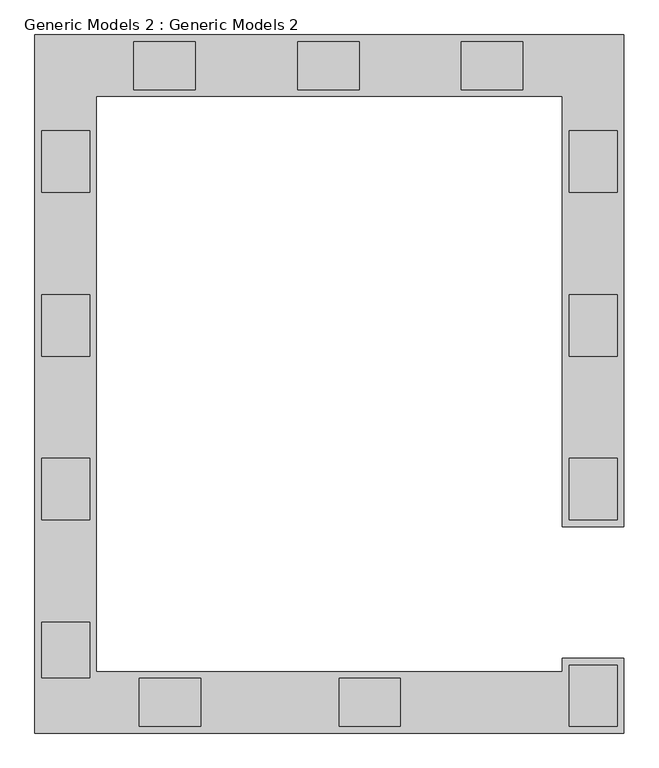
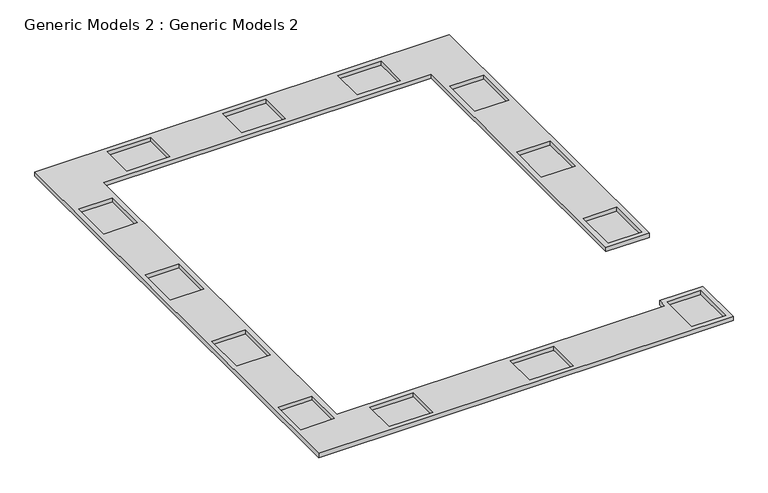
"""IFC4 building model written with IfcOpenShell, lengths in millimetres: proxy geometry, Generic Models 2 : Generic Models 2."""

from ifc_helpers import new_model, si_unit, origin, place, context, project, spatial, faceted_brep, source, transform, mapped, element, save


def generic_models_2_generic_models_2_55b91b29(model_context):
    return source(origin(), model_context, "Body", "Brep", [
        faceted_brep([(3323.8722402, 14495.4342801, 37.3542959), (-14214.8277598, 14495.4342801, 37.3542959), (-14214.8277598, -6294.4657199, 37.3542959), (3323.8722402, -6294.4657199, 37.3542959), (3323.8722402, -4071.9657199, 37.3542959), (1495.0722402, -4071.9657199, 37.3542959), (1495.0722402, -4465.6657199, 37.3542959), (-12386.0277598, -4465.6657199, 37.3542959), (-12386.0277598, 12666.6342801, 37.3542959), (1495.0722402, 12666.6342801, 37.3542959), (1495.0722402, -147.6657199, 37.3542959), (3323.8722402, -147.6657199, 37.3542959), (-12589.2277598, 11637.9342801, 37.3542959), (-12589.2277598, 9809.1342801, 37.3542959), (-14011.6277598, 9809.1342801, 37.3542959), (-14011.6277598, 11637.9342801, 37.3542959), (1698.2722402, -4668.8657199, 37.3542959), (1698.2722402, -4275.1657199, 37.3542959), (3120.6722402, -4275.1657199, 37.3542959), (3120.6722402, -6091.2657199, 37.3542959), (1698.2722402, -6091.2657199, 37.3542959), (-3330.9277598, -6091.2657199, 37.3542959), (-5159.7277598, -6091.2657199, 37.3542959), (-5159.7277598, -4668.8657199, 37.3542959), (-3330.9277598, -4668.8657199, 37.3542959), (-14011.6277598, -4644.0376355, 37.3542959), (-14011.6277598, -2992.4657199, 37.3542959), (-12589.2277598, -2992.4657199, 37.3542959), (-12589.2277598, -4644.0376355, 37.3542959), (-11268.4277598, 14292.2342801, 37.3542959), (-9439.6277598, 14292.2342801, 37.3542959), (-9439.6277598, 12869.8342801, 37.3542959), (-11268.4277598, 12869.8342801, 37.3542959), (3120.6722402, 11637.9342801, 37.3542959), (3120.6722402, 9809.1342801, 37.3542959), (1698.2722402, 9809.1342801, 37.3542959), (1698.2722402, 11637.9342801, 37.3542959), (3120.6722402, 55.5342801, 37.3542959), (1698.2722402, 55.5342801, 37.3542959), (1698.2722402, 1884.3342801, 37.3542959), (3120.6722402, 1884.3342801, 37.3542959), (313.9722402, 12869.8342801, 37.3542959), (-1514.8277598, 12869.8342801, 37.3542959), (-1514.8277598, 14292.2342801, 37.3542959), (313.9722402, 14292.2342801, 37.3542959), (1698.2722402, 4932.3342801, 37.3542959), (1698.2722402, 6761.1342801, 37.3542959), (3120.6722402, 6761.1342801, 37.3542959), (3120.6722402, 4932.3342801, 37.3542959), (-4562.8277598, 12869.8342801, 37.3542959), (-6391.6277598, 12869.8342801, 37.3542959), (-6391.6277598, 14292.2342801, 37.3542959), (-4562.8277598, 14292.2342801, 37.3542959), (-12589.2277598, 6761.1342801, 37.3542959), (-12589.2277598, 4932.3342801, 37.3542959), (-14011.6277598, 4932.3342801, 37.3542959), (-14011.6277598, 6761.1342801, 37.3542959), (-12589.2277598, 1884.3342801, 37.3542959), (-12589.2277598, 55.5342801, 37.3542959), (-14011.6277598, 55.5342801, 37.3542959), (-14011.6277598, 1884.3342801, 37.3542959), (-9274.5277598, -6091.2657199, 37.3542959), (-11103.3277598, -6091.2657199, 37.3542959), (-11103.3277598, -4668.8657199, 37.3542959), (-9274.5277598, -4668.8657199, 37.3542959), (3323.8722402, 14495.4342801, -152.4), (3323.8722402, -147.6657199, -152.4), (1495.0722402, -147.6657199, -152.4), (1495.0722402, 12666.6342801, -152.4), (-12386.0277598, 12666.6342801, -152.4), (-12386.0277598, -4465.6657199, -152.4), (1495.0722402, -4465.6657199, -152.4), (1495.0722402, -4071.9657199, -152.4), (3323.8722402, -4071.9657199, -152.4), (3323.8722402, -6294.4657199, -152.4), (-14214.8277598, -6294.4657199, -152.4), (-14214.8277598, 14495.4342801, -152.4), (-1514.8277598, 12869.8342801, -135.586224), (313.9722402, 12869.8342801, -135.586224), (313.9722402, 14292.2342801, -135.586224), (-1514.8277598, 14292.2342801, -135.586224), (1698.2722402, 1884.3342801, -135.586224), (1698.2722402, 55.5342801, -135.586224), (3120.6722402, 55.5342801, -135.586224), (3120.6722402, 1884.3342801, -135.586224), (3120.6722402, 9809.1342801, -135.586224), (3120.6722402, 11637.9342801, -135.586224), (1698.2722402, 11637.9342801, -135.586224), (1698.2722402, 9809.1342801, -135.586224), (-9439.6277598, 14292.2342801, -135.586224), (-11268.4277598, 14292.2342801, -135.586224), (-11268.4277598, 12869.8342801, -135.586224), (-9439.6277598, 12869.8342801, -135.586224), (-14011.6277598, -2992.4657199, -135.586224), (-14011.6277598, -4644.0376355, -135.586224), (-12589.2277598, -4644.0376355, -135.586224), (-12589.2277598, -2992.4657199, -135.586224), (-5159.7277598, -6091.2657199, -135.586224), (-3330.9277598, -6091.2657199, -135.586224), (-3330.9277598, -4668.8657199, -135.586224), (-5159.7277598, -4668.8657199, -135.586224), (3120.6722402, -6091.2657199, -135.586224), (3120.6722402, -4275.1657199, -135.586224), (1698.2722402, -4275.1657199, -135.586224), (1698.2722402, -4668.8657199, -135.586224), (1698.2722402, -6091.2657199, -135.586224), (-12589.2277598, 9809.1342801, -135.586224), (-12589.2277598, 11637.9342801, -135.586224), (-14011.6277598, 11637.9342801, -135.586224), (-14011.6277598, 9809.1342801, -135.586224), (1698.2722402, 4932.3342801, -135.586224), (3120.6722402, 4932.3342801, -135.586224), (3120.6722402, 6761.1342801, -135.586224), (1698.2722402, 6761.1342801, -135.586224), (-4562.8277598, 12869.8342801, -135.586224), (-4562.8277598, 14292.2342801, -135.586224), (-6391.6277598, 14292.2342801, -135.586224), (-6391.6277598, 12869.8342801, -135.586224), (-12589.2277598, 6761.1342801, -135.586224), (-14011.6277598, 6761.1342801, -135.586224), (-14011.6277598, 4932.3342801, -135.586224), (-12589.2277598, 4932.3342801, -135.586224), (-12589.2277598, 1884.3342801, -135.586224), (-14011.6277598, 1884.3342801, -135.586224), (-14011.6277598, 55.5342801, -135.586224), (-12589.2277598, 55.5342801, -135.586224), (-9274.5277598, -6091.2657199, -135.586224), (-9274.5277598, -4668.8657199, -135.586224), (-11103.3277598, -4668.8657199, -135.586224), (-11103.3277598, -6091.2657199, -135.586224)], [[[0, 1, 2, 3, 4, 5, 6, 7, 8, 9, 10, 11], [12, 13, 14, 15], [16, 17, 18, 19, 20], [21, 22, 23, 24], [25, 26, 27, 28], [29, 30, 31, 32], [33, 34, 35, 36], [37, 38, 39, 40], [41, 42, 43, 44], [45, 46, 47, 48], [49, 50, 51, 52], [53, 54, 55, 56], [57, 58, 59, 60], [61, 62, 63, 64]], [[65, 66, 67, 68, 69, 70, 71, 72, 73, 74, 75, 76]], [[1, 0, 65, 76]], [[2, 1, 76, 75]], [[3, 2, 75, 74]], [[0, 11, 66, 65]], [[10, 9, 68, 67]], [[7, 6, 71, 70]], [[8, 7, 70, 69]], [[9, 8, 69, 68]], [[4, 3, 74, 73]], [[5, 4, 73, 72]], [[6, 5, 72, 71]], [[11, 10, 67, 66]], [[77, 78, 79, 80]], [[81, 82, 83, 84]], [[85, 86, 87, 88]], [[89, 90, 91, 92]], [[93, 94, 95, 96]], [[97, 98, 99, 100]], [[101, 102, 103, 104, 105]], [[106, 107, 108, 109]], [[110, 111, 112, 113]], [[114, 115, 116, 117]], [[118, 119, 120, 121]], [[122, 123, 124, 125]], [[126, 127, 128, 129]], [[107, 106, 13, 12]], [[104, 103, 17, 16]], [[103, 102, 18, 17]], [[102, 101, 19, 18]], [[98, 97, 22, 21]], [[94, 93, 26, 25]], [[90, 89, 30, 29]], [[86, 85, 34, 33]], [[83, 82, 38, 37]], [[82, 81, 39, 38]], [[78, 77, 42, 41]], [[77, 80, 43, 42]], [[80, 79, 44, 43]], [[79, 78, 41, 44]], [[89, 92, 31, 30]], [[92, 91, 32, 31]], [[91, 90, 29, 32]], [[93, 96, 27, 26]], [[96, 95, 28, 27]], [[95, 94, 25, 28]], [[106, 109, 14, 13]], [[109, 108, 15, 14]], [[108, 107, 12, 15]], [[97, 100, 23, 22]], [[100, 99, 24, 23]], [[99, 98, 21, 24]], [[101, 105, 20, 19]], [[105, 104, 16, 20]], [[85, 88, 35, 34]], [[88, 87, 36, 35]], [[87, 86, 33, 36]], [[81, 84, 40, 39]], [[84, 83, 37, 40]], [[110, 113, 46, 45]], [[113, 112, 47, 46]], [[112, 111, 48, 47]], [[111, 110, 45, 48]], [[114, 117, 50, 49]], [[117, 116, 51, 50]], [[116, 115, 52, 51]], [[115, 114, 49, 52]], [[118, 121, 54, 53]], [[121, 120, 55, 54]], [[120, 119, 56, 55]], [[119, 118, 53, 56]], [[122, 125, 58, 57]], [[125, 124, 59, 58]], [[124, 123, 60, 59]], [[123, 122, 57, 60]], [[126, 129, 62, 61]], [[129, 128, 63, 62]], [[128, 127, 64, 63]], [[127, 126, 61, 64]]]),
    ])


if __name__ == "__main__":
    model = new_model("IFC4")
    model_context = context("Model", 3, world=origin())
    ifc_project = project(units=[si_unit("LENGTHUNIT", "METRE", prefix="MILLI")], contexts=[model_context])
    site = spatial("IfcSite", under=ifc_project)
    building = spatial("IfcBuilding", under=site)
    placement = place(None, origin())
    generic_models_2_generic_models_2_shape = generic_models_2_generic_models_2_55b91b29(model_context)
    element("IfcBuildingElementProxy", 1, Name="Generic Models 2 : Generic Models 2", ObjectType="Generic Models 2 : Generic Models 2", at=placement, inside=building, context=model_context, shape_type="MappedRepresentation", body=[
        mapped(generic_models_2_generic_models_2_shape, transform((0.0, 0.0, 0.0), x_axis=(1.0, 0.0, 0.0), y_axis=(0.0, 1.0, 0.0), z_axis=(0.0, 0.0, 1.0))),
    ])
    save(model, "model.ifc")
